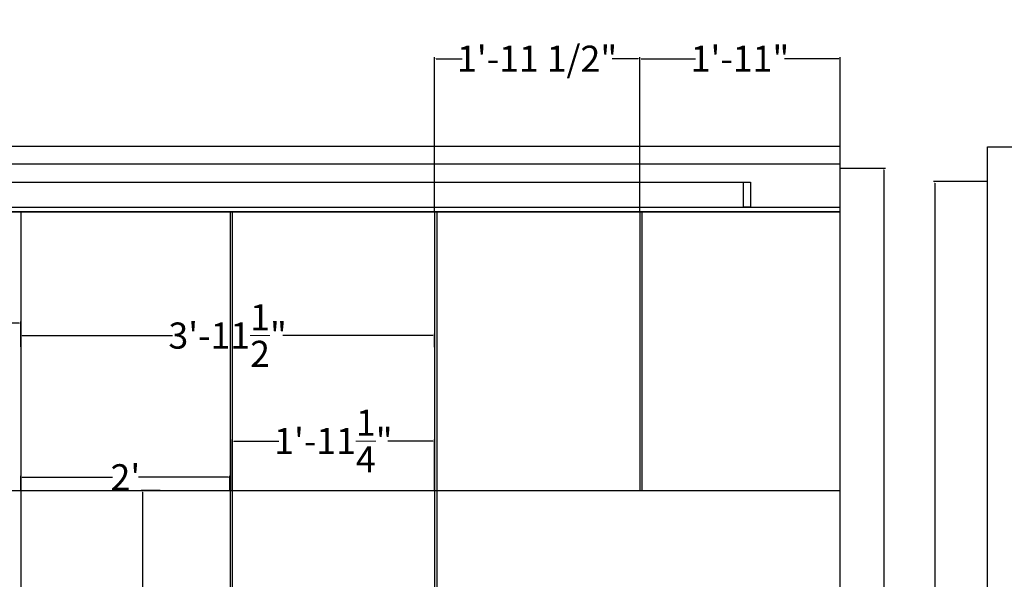
# Model space of a CAD drawing. Units: inches. Extents: x 1686244 to 1686928, y 1936095 to 1936489.
# Tile 6 of 11: x 1686365 to 1686478, y 1936425 to 1936489. Entities that reach past the tile are written whole.
import ezdxf

# ---------------------------------------------------------------- set-up
doc = ezdxf.new("R2010")
doc.units = ezdxf.units.IN
doc.header["$MEASUREMENT"] = 0
doc.layers.add('A-ANNO-DIMS', color=240, linetype='Continuous', lineweight=18)
doc.layers.add('A-ELEV', color=7, linetype='Continuous', lineweight=25)
doc.styles.get("Standard").update_dxf_attribs({"font": 'arial.ttf'})
doc.dimstyles.get("Standard").update_dxf_attribs({"dimtxt": 3, "dimasz": 0.18, "dimexe": 0.18, "dimexo": 0.0625, "dimgap": 0.09, "dimtad": 0, "dimtih": 1, "dimtoh": 1, "dimzin": 0, "dimdsep": 46, "dimlunit": 4, "dimtxsty": 'Standard', "dimcen": 0.09, "dimadec": 0, "dimazin": 0, "dimtfac": 1, "dimtofl": 0, "dimtmove": 0, "dimatfit": 3, "dimfxl": 1, "dimtolj": 1, "dimtzin": 0, "dimarcsym": 0})

# ---------------------------------------------------------------- blocks, each defined once
blk = doc.blocks.new('*D2')
at = {"layer": 'A-ANNO-DIMS', "color": 0, "lineweight": -2, "transparency": 16777216}
for p, q in [((1686365.35, 1936451.9), (1686365.35, 1936453.38)), ((1686365.53, 1936453.2), (1686382.75, 1936453.2)), ((1686412.63, 1936453.2), (1686395.42, 1936453.2)), ((1686412.81, 1936451.87), (1686412.81, 1936453.38))]:
    blk.add_line(p, q, dxfattribs=at)
at = {"layer": 'A-ANNO-DIMS', "color": 0, "transparency": 16777216}
for points in [[(1686365.53, 1936453.23), (1686365.53, 1936453.17), (1686365.35, 1936453.2)], [(1686412.63, 1936453.23), (1686412.63, 1936453.17), (1686412.81, 1936453.2)]]:
    blk.add_solid(points, dxfattribs=at)
at = {"layer": 'Defpoints', "color": 0, "transparency": 16777216}
for p in [(1686412.81, 1936453.2), (1686365.35, 1936451.84), (1686412.81, 1936451.81)]:
    blk.add_point(p, dxfattribs=at)
at = {"layer": 'A-ANNO-DIMS', "color": 0, "transparency": 16777216, "insert": (1686389.08, 1936453.2), "char_height": 3, "attachment_point": 5}
blk.add_mtext('\\A1;3\'-11{\\H1x;\\S1/2;}"', dxfattribs=at)
blk = doc.blocks.new('*D5')
at = {"layer": 'A-ANNO-DIMS', "color": 0, "lineweight": -2, "transparency": 16777216}
for p, q in [((1686321.85, 1936453.07), (1686321.85, 1936454.82)), ((1686322.03, 1936454.64), (1686338.43, 1936454.64)), ((1686365.17, 1936454.64), (1686348.77, 1936454.64)), ((1686365.35, 1936453.07), (1686365.35, 1936454.82))]:
    blk.add_line(p, q, dxfattribs=at)
at = {"layer": 'A-ANNO-DIMS', "color": 0, "transparency": 16777216}
for points in [[(1686322.03, 1936454.67), (1686322.03, 1936454.61), (1686321.85, 1936454.64)], [(1686365.17, 1936454.67), (1686365.17, 1936454.61), (1686365.35, 1936454.64)]]:
    blk.add_solid(points, dxfattribs=at)
at = {"layer": 'Defpoints', "color": 0, "transparency": 16777216}
for p in [(1686365.35, 1936454.64), (1686321.85, 1936453.01), (1686365.35, 1936453.01)]:
    blk.add_point(p, dxfattribs=at)
at = {"layer": 'A-ANNO-DIMS', "color": 0, "transparency": 16777216, "insert": (1686343.6, 1936454.64), "char_height": 3, "attachment_point": 5}
blk.add_mtext('\\A1;3\'-7{\\H1x;\\S1/2;}"', dxfattribs=at)
blk = doc.blocks.new('*D7')
at = {"layer": 'A-ANNO-DIMS', "color": 0, "lineweight": -2, "transparency": 16777216}
for p, q in [((1686365.35, 1936435.47), (1686365.35, 1936437.12)), ((1686365.53, 1936436.94), (1686375.86, 1936436.94)), ((1686389.17, 1936436.94), (1686378.85, 1936436.94)), ((1686389.35, 1936435.47), (1686389.35, 1936437.12))]:
    blk.add_line(p, q, dxfattribs=at)
at = {"layer": 'A-ANNO-DIMS', "color": 0, "transparency": 16777216}
for points in [[(1686365.53, 1936436.97), (1686365.53, 1936436.91), (1686365.35, 1936436.94)], [(1686389.17, 1936436.97), (1686389.17, 1936436.91), (1686389.35, 1936436.94)]]:
    blk.add_solid(points, dxfattribs=at)
at = {"layer": 'Defpoints', "color": 0, "transparency": 16777216}
for p in [(1686389.35, 1936436.94), (1686365.35, 1936435.41), (1686389.35, 1936435.41)]:
    blk.add_point(p, dxfattribs=at)
at = {"layer": 'A-ANNO-DIMS', "color": 0, "transparency": 16777216, "insert": (1686377.35, 1936436.94), "char_height": 3, "attachment_point": 5}
blk.add_mtext("\\A1;2'", dxfattribs=at)
blk = doc.blocks.new('*D8')
at = {"layer": 'A-ANNO-DIMS', "color": 0, "lineweight": -2, "transparency": 16777216}
for p, q in [((1686381.35, 1936435.41), (1686379.15, 1936435.41)), ((1686379.33, 1936435.23), (1686379.33, 1936398.03)), ((1686379.33, 1936357.59), (1686379.33, 1936394.79)), ((1686381.35, 1936357.41), (1686379.15, 1936357.41))]:
    blk.add_line(p, q, dxfattribs=at)
at = {"layer": 'A-ANNO-DIMS', "color": 0, "transparency": 16777216}
for points in [[(1686379.3, 1936435.23), (1686379.36, 1936435.23), (1686379.33, 1936435.41)], [(1686379.3, 1936357.59), (1686379.36, 1936357.59), (1686379.33, 1936357.41)]]:
    blk.add_solid(points, dxfattribs=at)
at = {"layer": 'Defpoints', "color": 0, "transparency": 16777216}
for p in [(1686379.33, 1936435.41), (1686381.41, 1936435.41), (1686381.41, 1936357.41)]:
    blk.add_point(p, dxfattribs=at)
at = {"layer": 'A-ANNO-DIMS', "color": 0, "transparency": 16777216, "insert": (1686379.33, 1936396.41), "char_height": 3, "attachment_point": 5}
blk.add_mtext('\\A1;6\'-6"', dxfattribs=at)
blk = doc.blocks.new('*D9')
at = {"layer": 'A-ANNO-DIMS', "color": 0, "lineweight": -2, "transparency": 16777216}
for p, q in [((1686389.61, 1936435.47), (1686389.61, 1936441.28)), ((1686389.79, 1936441.1), (1686394.97, 1936441.1)), ((1686412.63, 1936441.1), (1686407.45, 1936441.1)), ((1686412.81, 1936435.47), (1686412.81, 1936441.28))]:
    blk.add_line(p, q, dxfattribs=at)
at = {"layer": 'A-ANNO-DIMS', "color": 0, "transparency": 16777216}
for points in [[(1686389.79, 1936441.13), (1686389.79, 1936441.07), (1686389.61, 1936441.1)], [(1686412.63, 1936441.13), (1686412.63, 1936441.07), (1686412.81, 1936441.1)]]:
    blk.add_solid(points, dxfattribs=at)
at = {"layer": 'Defpoints', "color": 0, "transparency": 16777216}
for p in [(1686389.61, 1936441.1), (1686389.61, 1936435.41), (1686412.81, 1936435.41)]:
    blk.add_point(p, dxfattribs=at)
at = {"layer": 'A-ANNO-DIMS', "color": 0, "transparency": 16777216, "insert": (1686401.21, 1936441.1), "char_height": 3, "attachment_point": 5}
blk.add_mtext('\\A1;1\'-11{\\H1x;\\S1/4;}"', dxfattribs=at)
blk = doc.blocks.new('*D20')
at = {"layer": 'A-ANNO-DIMS', "color": 0, "lineweight": -2, "transparency": 16777216}
for p, q in [((1686476.2, 1936470.86), (1686470.03, 1936470.86)), ((1686470.21, 1936470.68), (1686470.21, 1936412.44)), ((1686470.21, 1936351.04), (1686470.21, 1936409.19)), ((1686476.2, 1936350.86), (1686470.03, 1936350.86))]:
    blk.add_line(p, q, dxfattribs=at)
at = {"layer": 'A-ANNO-DIMS', "color": 0, "transparency": 16777216}
for points in [[(1686470.18, 1936470.68), (1686470.24, 1936470.68), (1686470.21, 1936470.86)], [(1686470.18, 1936351.04), (1686470.24, 1936351.04), (1686470.21, 1936350.86)]]:
    blk.add_solid(points, dxfattribs=at)
at = {"layer": 'Defpoints', "color": 0, "transparency": 16777216}
for p in [(1686476.26, 1936470.86), (1686470.21, 1936350.86), (1686476.26, 1936350.86)]:
    blk.add_point(p, dxfattribs=at)
at = {"layer": 'A-ANNO-DIMS', "color": 0, "transparency": 16777216, "insert": (1686470.21, 1936410.81), "char_height": 3, "attachment_point": 5}
blk.add_mtext("\\A1;10'", dxfattribs=at)
blk = doc.blocks.new('*D64')
at = {"layer": 'A-ANNO-DIMS', "color": 0, "lineweight": -2, "transparency": 16777216}
for p, q in [((1686459.35, 1936472.41), (1686464.53, 1936472.41)), ((1686464.35, 1936472.23), (1686464.35, 1936414.03)), ((1686464.35, 1936352.59), (1686464.35, 1936410.79)), ((1686459.35, 1936352.41), (1686464.53, 1936352.41))]:
    blk.add_line(p, q, dxfattribs=at)
at = {"layer": 'A-ANNO-DIMS', "color": 0, "transparency": 16777216}
for points in [[(1686464.32, 1936472.23), (1686464.38, 1936472.23), (1686464.35, 1936472.41)], [(1686464.32, 1936352.59), (1686464.38, 1936352.59), (1686464.35, 1936352.41)]]:
    blk.add_solid(points, dxfattribs=at)
at = {"layer": 'Defpoints', "color": 0, "transparency": 16777216}
for p in [(1686459.29, 1936472.41), (1686459.29, 1936352.41), (1686464.35, 1936352.41)]:
    blk.add_point(p, dxfattribs=at)
at = {"layer": 'A-ANNO-DIMS', "color": 0, "transparency": 16777216, "insert": (1686464.35, 1936412.41), "char_height": 3, "attachment_point": 5}
blk.add_mtext("\\A1;10'", dxfattribs=at)
blk = doc.blocks.new('*D93')
at = {"layer": 'A-ANNO-DIMS', "color": 0, "lineweight": -2, "transparency": 16777216}
for p, q in [((1686412.81, 1936467.47), (1686412.81, 1936485.14)), ((1686436.35, 1936467.47), (1686436.35, 1936485.14)), ((1686412.99, 1936484.96), (1686415.98, 1936484.96)), ((1686436.17, 1936484.96), (1686433.18, 1936484.96))]:
    blk.add_line(p, q, dxfattribs=at)
at = {"layer": 'A-ANNO-DIMS', "color": 0, "transparency": 16777216}
for points in [[(1686412.99, 1936484.99), (1686412.99, 1936484.93), (1686412.81, 1936484.96)], [(1686436.17, 1936484.99), (1686436.17, 1936484.93), (1686436.35, 1936484.96)]]:
    blk.add_solid(points, dxfattribs=at)
at = {"layer": 'Defpoints', "color": 0, "transparency": 16777216}
for p in [(1686436.35, 1936484.96), (1686412.81, 1936467.41), (1686436.35, 1936467.41)]:
    blk.add_point(p, dxfattribs=at)
at = {"layer": 'A-ANNO-DIMS', "color": 0, "transparency": 16777216, "insert": (1686424.58, 1936484.96), "char_height": 3, "attachment_point": 5}
blk.add_mtext('\\A1;1\'-11 1/2"', dxfattribs=at)
blk = doc.blocks.new('*D94')
at = {"layer": 'A-ANNO-DIMS', "color": 0, "lineweight": -2, "transparency": 16777216}
for p, q in [((1686436.35, 1936467.47), (1686436.35, 1936485.14)), ((1686459.35, 1936467.47), (1686459.35, 1936485.14)), ((1686436.53, 1936484.96), (1686442.75, 1936484.96)), ((1686459.17, 1936484.96), (1686452.95, 1936484.96))]:
    blk.add_line(p, q, dxfattribs=at)
at = {"layer": 'A-ANNO-DIMS', "color": 0, "transparency": 16777216}
for points in [[(1686436.53, 1936484.99), (1686436.53, 1936484.93), (1686436.35, 1936484.96)], [(1686459.17, 1936484.99), (1686459.17, 1936484.93), (1686459.35, 1936484.96)]]:
    blk.add_solid(points, dxfattribs=at)
at = {"layer": 'Defpoints', "color": 0, "transparency": 16777216}
for p in [(1686459.35, 1936484.96), (1686436.35, 1936467.41), (1686459.35, 1936467.41)]:
    blk.add_point(p, dxfattribs=at)
at = {"layer": 'A-ANNO-DIMS', "color": 0, "transparency": 16777216, "insert": (1686447.85, 1936484.96), "char_height": 3, "attachment_point": 5}
blk.add_mtext('\\A1;1\'-11"', dxfattribs=at)

msp = doc.modelspace()

# ---------------------------------------------------------------- linework, layer by layer
at = {"layer": 'A-ELEV'}
for p, q in [((1686262.353, 1936474.912), (1686459.353, 1936474.912)), ((1686459.353, 1936467.412), (1686459.353, 1936474.912)), ((1686262.353, 1936472.912), (1686459.353, 1936472.912)), ((1686282.448, 1936470.78), (1686449.069, 1936470.78)), ((1686448.259, 1936467.912), (1686448.259, 1936470.78)), ((1686449.069, 1936470.78), (1686449.069, 1936467.912)), ((1686262.353, 1936467.912), (1686459.353, 1936467.912)), ((1686262.353, 1936467.412), (1686459.353, 1936467.412)), ((1686365.353, 1936467.412), (1686365.353, 1936357.412)), ((1686389.353, 1936467.412), (1686389.353, 1936357.412)), ((1686389.609, 1936467.412), (1686389.609, 1936357.412)), ((1686412.809, 1936467.412), (1686412.809, 1936357.412)), ((1686413.059, 1936467.412), (1686413.059, 1936357.412)), ((1686436.353, 1936467.412), (1686436.353, 1936435.412)), ((1686436.603, 1936467.412), (1686436.603, 1936435.412)), ((1686449.069, 1936467.912), (1686448.259, 1936467.912)), ((1686262.353, 1936435.412), (1686459.353, 1936435.412))]:
    msp.add_line(p, q, dxfattribs=at)
for points in [[(1686691.259, 1936346.864), (1686476.258, 1936346.864), (1686476.258, 1936474.864), (1686691.259, 1936474.864)], [(1686459.353, 1936357.412), (1686459.353, 1936467.412), (1686262.353, 1936467.412), (1686262.353, 1936357.412)]]:
    msp.add_lwpolyline(points, close=True, dxfattribs=at)

# ---------------------------------------------------------------- dimensions: what is measured, and where the dimension line sits
at = {"layer": 'A-ANNO-DIMS'}
for base, p1, p2, override, picture, middle in [((1686436.353, 1936484.962), (1686412.809, 1936467.412), (1686436.353, 1936467.412), {"dimdec": 1, "dimlfac": 1, "dimrnd": 0, "dimzin": 1, "dimdsep": 46, "dimlunit": 4, "dimfrac": 2}, '*D93', (1686424.581, 1936484.962)), ((1686459.353, 1936484.962), (1686436.353, 1936467.412), (1686459.353, 1936467.412), {"dimdec": 1, "dimlfac": 1, "dimrnd": 0, "dimzin": 1, "dimdsep": 46, "dimlunit": 4, "dimfrac": 2}, '*D94', (1686447.853, 1936484.962)), ((1686365.353, 1936454.64), (1686321.853, 1936453.01), (1686365.353, 1936453.01), {"dimclrd": 0, "dimclre": 0, "dimclrt": 0}, '*D5', (1686343.603, 1936454.64)), ((1686412.809, 1936453.199), (1686365.353, 1936451.84), (1686412.809, 1936451.81), {"dimclrd": 0, "dimclre": 0, "dimclrt": 0}, '*D2', (1686389.081, 1936453.199)), ((1686389.609, 1936441.098), (1686412.809, 1936435.412), (1686389.609, 1936435.412), {"dimclrd": 0, "dimclre": 0, "dimclrt": 0}, '*D9', (1686401.209, 1936441.098)), ((1686389.353, 1936436.944), (1686365.353, 1936435.412), (1686389.353, 1936435.412), {"dimclrd": 0, "dimclre": 0, "dimclrt": 0}, '*D7', (1686377.353, 1936436.944))]:
    dim = msp.add_linear_dim(base=base, p1=p1, p2=p2, dimstyle='Standard', override=override, dxfattribs=at)
    dim.commit()
    dim.dimension.update_dxf_attribs({"geometry": picture, "text_midpoint": middle})
for base, p1, p2, picture, middle in [((1686464.354, 1936352.412), (1686459.29, 1936472.412), (1686459.29, 1936352.412), '*D64', (1686464.354, 1936412.412)), ((1686470.215, 1936350.864), (1686476.258, 1936470.864), (1686476.258, 1936350.864), '*D20', (1686470.215, 1936410.814))]:
    dim = msp.add_linear_dim(base=base, p1=p1, p2=p2, angle=90, dimstyle='Standard', override={"dimclrd": 0, "dimclre": 0, "dimclrt": 0}, dxfattribs=at)
    dim.commit()
    dim.dimension.update_dxf_attribs({"geometry": picture, "text_midpoint": middle, "dimtype": 160})
dim = msp.add_linear_dim(base=(1686379.328, 1936435.412), p1=(1686381.411, 1936357.412), p2=(1686381.411, 1936435.412), angle=90, dimstyle='Standard', override={"dimclrd": 0, "dimclre": 0, "dimclrt": 0}, dxfattribs=at)
dim.commit()
dim.dimension.update_dxf_attribs({"geometry": '*D8', "text_midpoint": (1686379.328, 1936396.412)})

doc.saveas('drawing.dxf')
